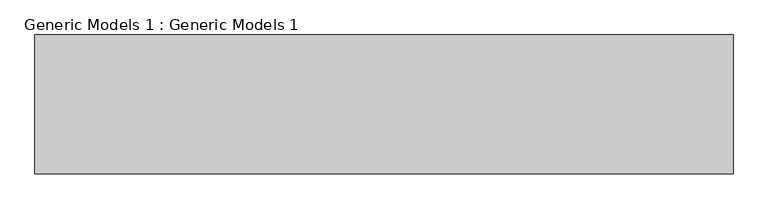
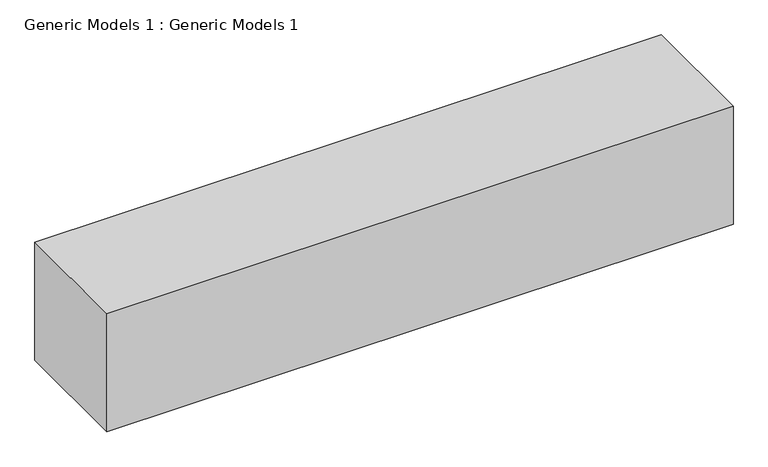
"""IFC4 building model written with IfcOpenShell, lengths in millimetres: proxy geometry, Generic Models 1 : Generic Models 1."""

from ifc_helpers import new_model, si_unit, frame, origin, place, context, project, spatial, polyline, outline, extrude, source, transform, mapped, element, save


def generic_models_1_generic_models_1_d7d81bca(model_context):
    return source(origin(), model_context, "Body", "SweptSolid", [
        extrude(outline(polyline([(-1792.7942549, -8570.658484), (-4855.6350579, -8570.658484), (-4855.6350579, -7961.058484), (-1792.7942549, -7961.058484), (-1792.7942549, -8570.658484)])), frame((0.0, 0.0, 2743.2), z_axis=(0.0, 0.0, 1.0), x_axis=(1.0, 0.0, 0.0)), (0.0, 0.0, 1.0), 609.6),
    ])


if __name__ == "__main__":
    model = new_model("IFC4")
    model_context = context("Model", 3, world=origin())
    ifc_project = project(units=[si_unit("LENGTHUNIT", "METRE", prefix="MILLI")], contexts=[model_context])
    site = spatial("IfcSite", under=ifc_project)
    building = spatial("IfcBuilding", under=site)
    placement = place(None, origin())
    generic_models_1_generic_models_1_shape = generic_models_1_generic_models_1_d7d81bca(model_context)
    element("IfcBuildingElementProxy", 1, Name="Generic Models 1 : Generic Models 1", ObjectType="Generic Models 1 : Generic Models 1", at=placement, inside=building, context=model_context, shape_type="MappedRepresentation", body=[
        mapped(generic_models_1_generic_models_1_shape, transform((0.0, 0.0, 0.0), x_axis=(1.0, 0.0, 0.0), y_axis=(0.0, 1.0, 0.0), z_axis=(0.0, 0.0, 1.0))),
    ])
    save(model, "model.ifc")
